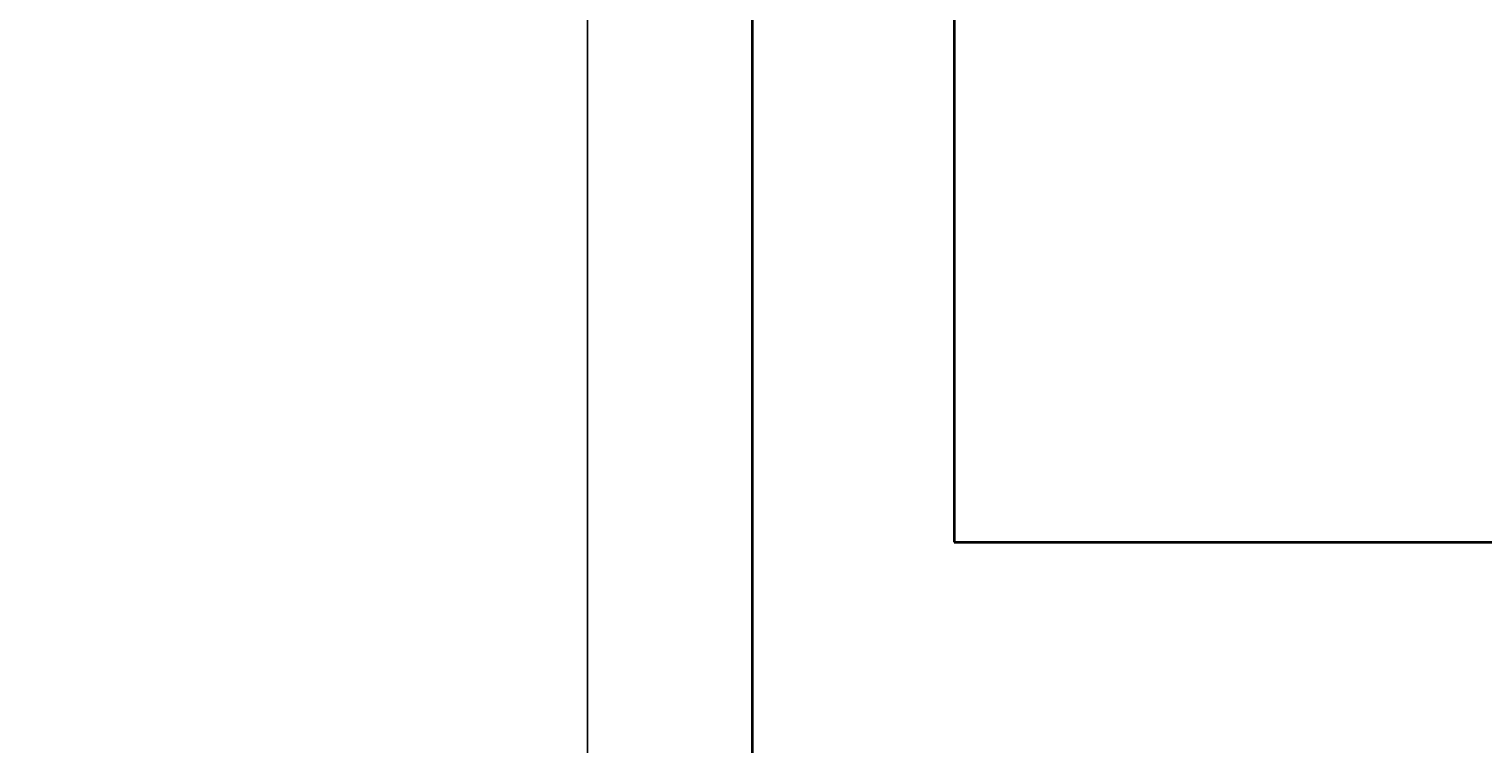
# Model space of a CAD drawing. Units: feet. Extents: x 5816 to 6644, y 25475 to 26788.
# Tile 17 of 23: x 6082 to 6147, y 26499 to 26530. Entities that reach past the tile are written whole.
import ezdxf

# ---------------------------------------------------------------- set-up
doc = ezdxf.new("R2010")
doc.units = ezdxf.units.FT
doc.layers.add('A-ANNO-DIMS', color=2, linetype='Continuous', lineweight=13)
doc.layers.add('A-WALL', color=7, linetype='Continuous', lineweight=35)
doc.styles.get("Standard").update_dxf_attribs({"font": 'arial.ttf'})
doc.dimstyles.get("Standard").update_dxf_attribs({"dimtxt": 0.18, "dimasz": 0.18, "dimexe": 0.18, "dimexo": 0.0625, "dimgap": 0.09, "dimtad": 0, "dimtih": 1, "dimtoh": 1, "dimdec": 4, "dimzin": 0, "dimdsep": 46, "dimtxsty": 'Standard', "dimcen": 0.09, "dimadec": 0, "dimazin": 0, "dimtfac": 1, "dimtdec": 4, "dimtofl": 0, "dimtmove": 0, "dimatfit": 3, "dimfxl": 1, "dimtolj": 1, "dimtzin": 0, "dimarcsym": 0})

# ---------------------------------------------------------------- blocks, each defined once
blk = doc.blocks.new('*D58')
at = {"layer": 'A-ANNO-DIMS', "color": 0, "lineweight": -2, "transparency": 16777216}
for p, q in [((5953.978, 26168.647), (5953.978, 26787.915)), ((5954.158, 26787.735), (6030.198, 26787.735)), ((6106.798, 26787.735), (6030.759, 26787.735)), ((6106.978, 26168.713), (6106.978, 26787.915))]:
    blk.add_line(p, q, dxfattribs=at)
at = {"layer": 'A-ANNO-DIMS', "color": 0, "transparency": 16777216}
for points in [[(5954.158, 26787.765), (5954.158, 26787.705), (5953.978, 26787.735)], [(6106.798, 26787.765), (6106.798, 26787.705), (6106.978, 26787.735)]]:
    blk.add_solid(points, dxfattribs=at)
at = {"layer": 'Defpoints', "color": 0, "transparency": 16777216}
for p in [(6106.978, 26787.735), (5953.978, 26168.585), (6106.978, 26168.651)]:
    blk.add_point(p, dxfattribs=at)
at = {"layer": 'A-ANNO-DIMS', "color": 0, "transparency": 16777216, "insert": (6030.478, 26787.735), "char_height": 0.18, "attachment_point": 5}
blk.add_mtext('\\A1;153', dxfattribs=at)
blk = doc.blocks.new('*D60')
at = {"layer": 'A-ANNO-DIMS', "color": 0, "lineweight": -2, "transparency": 16777216}
for p, q in [((6106.978, 26094.399), (6106.978, 26787.915)), ((6107.158, 26787.735), (6224.932, 26787.735)), ((6343.496, 26787.735), (6225.722, 26787.735)), ((6343.676, 26094.399), (6343.676, 26787.915))]:
    blk.add_line(p, q, dxfattribs=at)
at = {"layer": 'A-ANNO-DIMS', "color": 0, "transparency": 16777216}
for points in [[(6107.158, 26787.765), (6107.158, 26787.705), (6106.978, 26787.735)], [(6343.496, 26787.765), (6343.496, 26787.705), (6343.676, 26787.735)]]:
    blk.add_solid(points, dxfattribs=at)
at = {"layer": 'Defpoints', "color": 0, "transparency": 16777216}
for p in [(6343.676, 26787.735), (6106.978, 26094.337), (6343.676, 26094.337)]:
    blk.add_point(p, dxfattribs=at)
at = {"layer": 'A-ANNO-DIMS', "color": 0, "transparency": 16777216, "insert": (6225.327, 26787.735), "char_height": 0.18, "attachment_point": 5}
blk.add_mtext('\\A1;236.7', dxfattribs=at)

msp = doc.modelspace()

# ---------------------------------------------------------------- linework, layer by layer
at = {"layer": 'A-WALL'}
for p, q in [((6114.3119, 26558.5846), (6114.3119, 26491.3288)), ((6123.3119, 26558.5846), (6123.3119, 26507.5846)), ((6123.3119, 26507.5846), (6225.3119, 26507.5846))]:
    msp.add_line(p, q, dxfattribs=at)

# ---------------------------------------------------------------- dimensions: what is measured, and where the dimension line sits
at = {"layer": 'A-ANNO-DIMS'}
for base, p1, p2, override, picture, middle in [((6106.9781, 26787.7346), (5953.9781, 26168.5846), (6106.9781, 26168.6509), {"dimdec": 0, "dimlfac": 1, "dimrnd": 0, "dimzin": 0, "dimdsep": 46, "dimlunit": 2}, '*D58', (6030.4781, 26787.7346)), ((6343.6763, 26787.7346), (6106.9781, 26094.3368), (6343.6763, 26094.3368), {"dimdec": 1, "dimlfac": 1, "dimrnd": 0, "dimzin": 0, "dimdsep": 46, "dimlunit": 2}, '*D60', (6225.3272, 26787.7346))]:
    dim = msp.add_linear_dim(base=base, p1=p1, p2=p2, dimstyle='Standard', override=override, dxfattribs=at)
    dim.commit()
    dim.dimension.update_dxf_attribs({"geometry": picture, "text_midpoint": middle})

doc.saveas('drawing.dxf')
